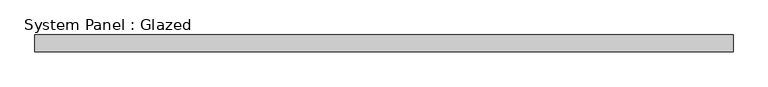
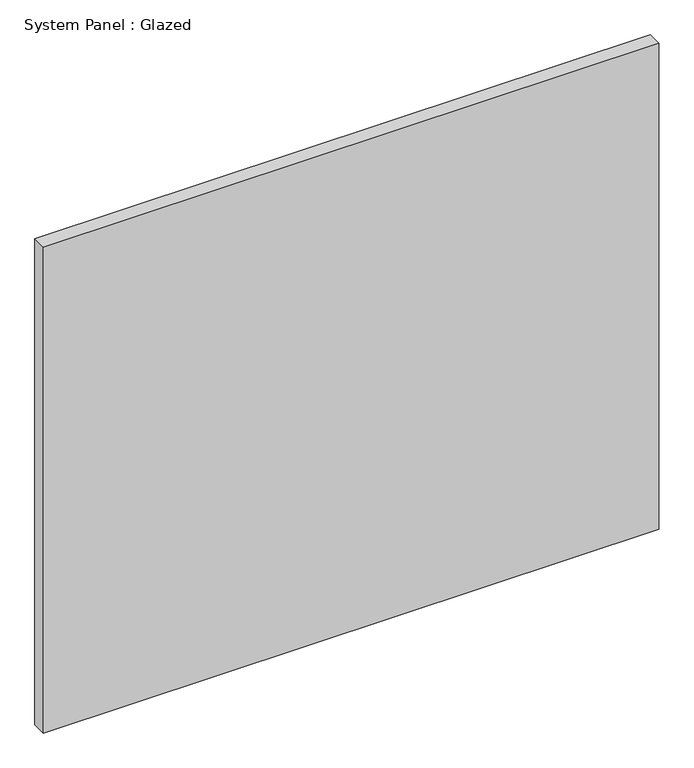
"""IFC4 building model written with IfcOpenShell, lengths in millimetres: plate geometry, System Panel : Glazed."""

from ifc_helpers import new_model, si_unit, origin, origin_with_axes, place, context, project, spatial, polyline, outline, extrude, source, transform, mapped, element, save


def system_panel_glazed_4a7c210e(model_context):
    return source(origin(), model_context, "Body", "SweptSolid", [
        extrude(outline(polyline([(533.4, 19.05), (-533.4, 19.05), (-533.4, 44.45), (533.4, 44.45), (533.4, 19.05)])), origin_with_axes(), (0.0, 0.0, 1.0), 890.5158113),
    ])


if __name__ == "__main__":
    model = new_model("IFC4")
    model_context = context("Model", 3, world=origin())
    ifc_project = project(units=[si_unit("LENGTHUNIT", "METRE", prefix="MILLI")], contexts=[model_context])
    site = spatial("IfcSite", under=ifc_project)
    building = spatial("IfcBuilding", under=site)
    placement = place(None, origin())
    system_panel_glazed_shape = system_panel_glazed_4a7c210e(model_context)
    element("IfcPlate", 1, ObjectType="System Panel : Glazed", at=placement, inside=building, context=model_context, shape_type="MappedRepresentation", body=[
        mapped(system_panel_glazed_shape, transform((0.0, 0.0, 0.0), x_axis=(1.0, 0.0, 0.0), y_axis=(0.0, 1.0, 0.0), z_axis=(0.0, 0.0, 1.0))),
    ])
    save(model, "model.ifc")

# Revit data of these elements
# Type "System Panel : Glazed"
#   Construction Type Id = "GSP4R"
#   Analytic Construction = "1/8 in Pilkington single glazing"
#   Visual Light Transmittance = 0.9
#   Solar Heat Gain Coefficient = 0.86
#   Heat Transfer Coefficient (U) = 1.18115 BTU/(h·ft²·°F)
#   Define Thermal Properties by = 1
# Element 1 (IfcPlate, "System Panel : Glazed")
#   Materials on its faces: "Glass"
# Materials
#   "Glass": class "Glass", colour RGB 0 128 192, transparency 0.75, Description = "Soda Lime Glass", Cost = 0
